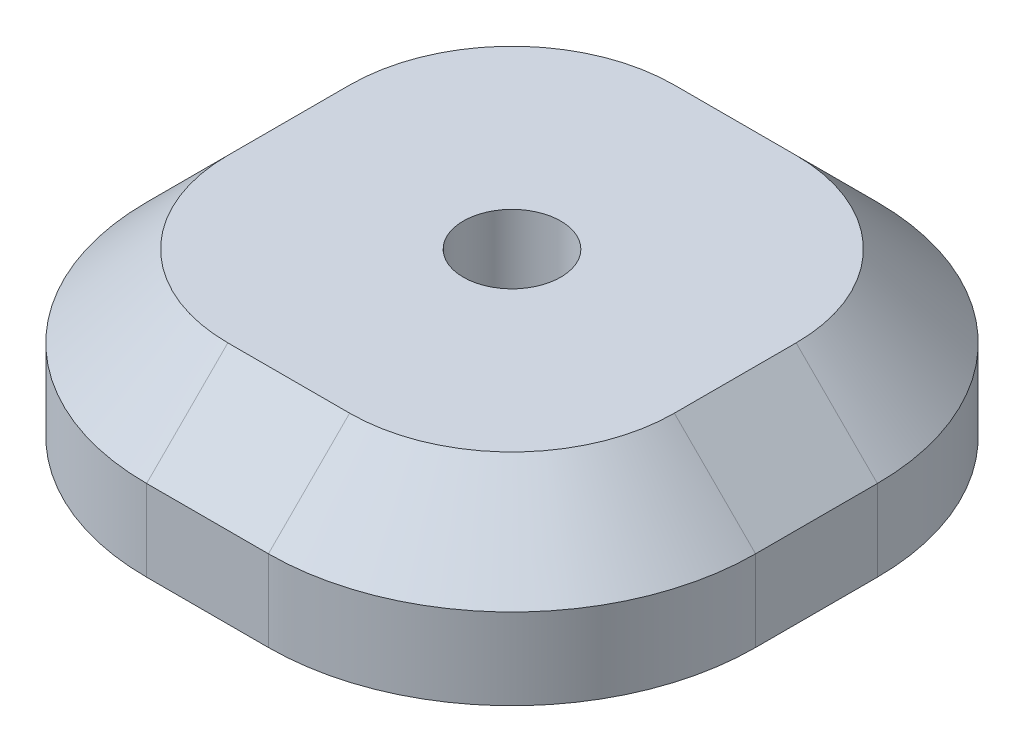
SolidWorks part; units mm, degrees
material "Plain Carbon Steel"
ref_plane "Front Plane" through (0, 0, 0) normal (0, 0, 1) x (1, 0, 0)
ref_plane "Top Plane" through (0, 0, 0) normal (0, 1, 0) x (1, 0, 0)
ref_plane "Right Plane" through (0, 0, 0) normal (1, 0, 0) x (0, 0, -1)
sketch "Base Profile Sketch 75x75" plane through (0, 0, 0) normal (0, 1, 0) x (1, 0, 0)
  line L1 (-37.5, -37.5) -> (37.5, -37.5)
  line L2 (-37.5, -37.5) -> (-37.5, 37.5)
  line L3 (-37.5, 37.5) -> (37.5, 37.5)
  line L4 (37.5, -37.5) -> (37.5, 37.5)
  line L5 (-37.5, -37.5) -> (37.5, 37.5) construction
  line L6 (-37.5, 37.5) -> (37.5, -37.5) construction
  point P0 (0, 0)
  dimension "D1" = 75
  dimension "D2" = 75
extrude "Base Block 75x75x20" add sketch "Base Profile Sketch 75x75" along normal blind 20
fillet "Corner Fillets R30" radius 30 4 edges at (-37.5, 10, -37.5) (37.5, 10, -37.5) (37.5, 10, 37.5) (-37.5, 10, 37.5)
chamfer "Top Edge Chamfer 10x45deg" distance 10 angle 45 8 edges at (0, 20, -37.5) (-28.7132, 20, -28.7132) (28.7132, 20, -28.7132) (-37.5, 20, 0) (37.5, 20, 0) (-28.7132, 20, 28.7132) (28.7132, 20, 28.7132) (0, 20, 37.5)
hole_wizard "Dowel Hole A Ø12x10" positions "3DSketch1" profile "Sketch3" hole size "Ø12.0" standard "ANSI Metric"
sketch3d "3DSketch1"
  point P0 (0, 20, 0)
sketch "Sketch3" plane through (0, 20, 0) normal (1, 0, 0) x (0, 0, 1)
  line L0 (0, 0) -> (0, 13.6052)
  line L1 (0, 13.6052) -> (6, 10)
  line L2 (6, 10) -> (6, 0)
  line L5 (6, 0) -> (0, 0)
  line L10 (0, 13.6052) -> (-6, 10) construction
  line L11 (0, -6.35) -> (0, 107.95) construction
  dimension "Hole Dia." = 12
  dimension "Hole Depth" = 10
  dimension "Drill Angle" = 118
sketch "Dowel Hole B Locator Sketch 25x25" plane through (0, 0, 0) normal (0, -1, 0) x (1, 0, 0)
  line L1 (-12.5, -12.5) -> (12.5, -12.5)
  line L2 (-12.5, -12.5) -> (-12.5, 12.5)
  line L3 (-12.5, 12.5) -> (12.5, 12.5)
  line L4 (12.5, -12.5) -> (12.5, 12.5)
  line L5 (-12.5, -12.5) -> (12.5, 12.5) construction
  line L6 (-12.5, 12.5) -> (12.5, -12.5) construction
  point P0 (0, 0)
  dimension "D1" = 25
  dimension "D2" = 25
hole_wizard "Dowel Hole B Ø12x10" positions "3DSketch2" profile "Sketch5" hole size "Ø12.0" standard "ANSI Metric"
sketch3d "3DSketch2"
  point P0 (-12.5, 0, 12.5)
  point P3 (12.5, 0, 12.5)
  point P6 (12.5, 0, -12.5)
  point P9 (-12.5, 0, -12.5)
sketch "Sketch5" plane through (-12.5, 0, 12.5) normal (1, 0, 0) x (0, 0, -1)
  line L0 (0, 0) -> (0, 13.6052)
  line L1 (0, 13.6052) -> (6, 10)
  line L2 (6, 10) -> (6, 0)
  line L5 (6, 0) -> (0, 0)
  line L10 (0, 13.6052) -> (-6, 10) construction
  line L11 (0, -6.35) -> (0, 107.95) construction
  dimension "Hole Dia." = 12
  dimension "Hole Depth" = 10
  dimension "Drill Angle" = 118
